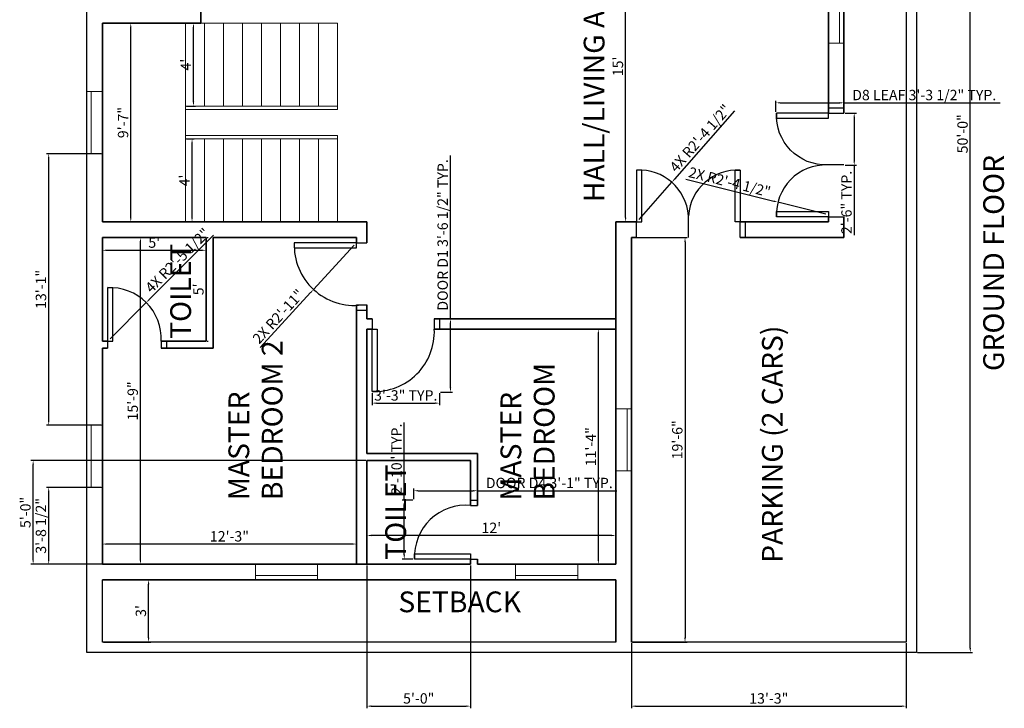
# Model space of a CAD drawing. Units: inches. Extents: x 2641 to 3210, y 2696 to 4064.
# Tile 1 of 4: x 2641 to 3210, y 2696 to 3095. Entities that reach past the tile are written whole.
import ezdxf

# ---------------------------------------------------------------- set-up
doc = ezdxf.new("R2010")
doc.units = ezdxf.units.IN
for name, color, linetype, lineweight in [('A-ANNO-DIMS', 2, 'Continuous', 18), ('A-ANNO-TEXT', 7, 'Continuous', 25), ('A-AREA-IDEN', 7, 'Continuous', 18), ('A-DOOR', 3, 'Continuous', 25), ('A-FLOR-STRS', 7, 'Continuous', 18), ('A-GLAZ', 4, 'Continuous', 18), ('A-WALL', 7, 'Continuous', 35), ('C-PROP', 8, 'Continuous', 25)]:
    doc.layers.add(name, color=color, linetype=linetype, lineweight=lineweight)
doc.styles.get("Standard").update_dxf_attribs({"font": 'arial.ttf'})
doc.dimstyles.new('ISO-25', dxfattribs={"dimtxt": 6, "dimasz": 2.5, "dimexe": 1.25, "dimexo": 0.625, "dimtad": 1, "dimdec": 1, "dimlunit": 3, "dimtxsty": 'Standard', "dimcen": 2.5, "dimadec": 0, "dimazin": 0, "dimtfac": 1, "dimtdec": 1, "dimtmove": 0, "dimatfit": 3, "dimfxl": 1, "dimarcsym": 0})

# ---------------------------------------------------------------- blocks, each defined once
blk = doc.blocks.new('*D2')
at = {"layer": 'A-ANNO-DIMS', "color": 0, "lineweight": -2, "transparency": 16777216}
for p, q in [((2689.25, 2968.55), (2711.9, 2968.55)), ((2710.65, 2782.05), (2710.65, 2966.05)), ((2689.25, 2779.55), (2711.9, 2779.55))]:
    blk.add_line(p, q, dxfattribs=at)
at = {"layer": 'A-ANNO-DIMS', "color": 0, "transparency": 16777216}
for points in [[(2710.23, 2966.05), (2711.06, 2966.05), (2710.65, 2968.55)], [(2710.23, 2782.05), (2711.06, 2782.05), (2710.65, 2779.55)]]:
    blk.add_solid(points, dxfattribs=at)
at = {"layer": 'Defpoints', "color": 0, "transparency": 16777216}
for p in [(2688.63, 2968.55), (2710.65, 2968.55), (2688.63, 2779.55)]:
    blk.add_point(p, dxfattribs=at)
at = {"layer": 'A-ANNO-DIMS', "color": 0, "transparency": 16777216, "insert": (2706.96, 2874.05), "char_height": 6, "attachment_point": 5, "rotation": 90}
blk.add_mtext('15\'-9"', dxfattribs=at)
blk = doc.blocks.new('*D3')
at = {"layer": 'A-ANNO-DIMS', "color": 0, "lineweight": -2, "transparency": 16777216}
for p, q in [((2688.63, 2780.17), (2688.63, 2792.51)), ((2833.13, 2791.26), (2691.13, 2791.26)), ((2835.63, 2780.17), (2835.63, 2792.51))]:
    blk.add_line(p, q, dxfattribs=at)
at = {"layer": 'A-ANNO-DIMS', "color": 0, "transparency": 16777216}
for points in [[(2691.13, 2791.68), (2691.13, 2790.85), (2688.63, 2791.26)], [(2833.13, 2791.68), (2833.13, 2790.85), (2835.63, 2791.26)]]:
    blk.add_solid(points, dxfattribs=at)
at = {"layer": 'Defpoints', "color": 0, "transparency": 16777216}
for p in [(2688.63, 2791.26), (2688.63, 2779.55), (2835.63, 2779.55)]:
    blk.add_point(p, dxfattribs=at)
at = {"layer": 'A-ANNO-DIMS', "color": 0, "transparency": 16777216, "insert": (2762.13, 2794.95), "char_height": 6, "attachment_point": 5}
blk.add_mtext('12\'-3"', dxfattribs=at)
blk = doc.blocks.new('*D4')
at = {"layer": 'A-ANNO-DIMS', "color": 0, "lineweight": -2, "transparency": 16777216}
for p, q in [((2841.63, 2780.17), (2841.63, 2797.47)), ((2985.63, 2780.17), (2985.63, 2797.47)), ((2983.13, 2796.22), (2844.13, 2796.22))]:
    blk.add_line(p, q, dxfattribs=at)
at = {"layer": 'A-ANNO-DIMS', "color": 0, "transparency": 16777216}
for points in [[(2844.13, 2796.64), (2844.13, 2795.8), (2841.63, 2796.22)], [(2983.13, 2796.64), (2983.13, 2795.8), (2985.63, 2796.22)]]:
    blk.add_solid(points, dxfattribs=at)
at = {"layer": 'Defpoints', "color": 0, "transparency": 16777216}
for p in [(2841.63, 2796.22), (2841.63, 2779.55), (2985.63, 2779.55)]:
    blk.add_point(p, dxfattribs=at)
at = {"layer": 'A-ANNO-DIMS', "color": 0, "transparency": 16777216, "insert": (2913.63, 2799.86), "char_height": 6, "attachment_point": 5}
blk.add_mtext("12'", dxfattribs=at)
blk = doc.blocks.new('*D5')
at = {"layer": 'A-ANNO-DIMS', "color": 0, "lineweight": -2, "transparency": 16777216}
for p, q in [((2985, 2915.55), (2974.29, 2915.55)), ((2975.54, 2782.05), (2975.54, 2913.05)), ((2985, 2779.55), (2974.29, 2779.55))]:
    blk.add_line(p, q, dxfattribs=at)
at = {"layer": 'A-ANNO-DIMS', "color": 0, "transparency": 16777216}
for points in [[(2975.13, 2913.05), (2975.96, 2913.05), (2975.54, 2915.55)], [(2975.13, 2782.05), (2975.96, 2782.05), (2975.54, 2779.55)]]:
    blk.add_solid(points, dxfattribs=at)
at = {"layer": 'Defpoints', "color": 0, "transparency": 16777216}
for p in [(2975.54, 2915.55), (2985.63, 2915.55), (2985.63, 2779.55)]:
    blk.add_point(p, dxfattribs=at)
at = {"layer": 'A-ANNO-DIMS', "color": 0, "transparency": 16777216, "insert": (2971.91, 2847.55), "char_height": 6, "attachment_point": 5, "rotation": 90}
blk.add_mtext('11\'-4"', dxfattribs=at)
blk = doc.blocks.new('*D6')
at = {"layer": 'A-ANNO-DIMS', "color": 0, "lineweight": -2, "transparency": 16777216}
for p, q in [((2749.25, 2968.55), (2749.88, 2968.55)), ((2748.63, 2911.05), (2748.63, 2966.05)), ((2749.25, 2908.55), (2749.88, 2908.55))]:
    blk.add_line(p, q, dxfattribs=at)
at = {"layer": 'A-ANNO-DIMS', "color": 0, "transparency": 16777216}
for points in [[(2748.21, 2966.05), (2749.04, 2966.05), (2748.63, 2968.55)], [(2748.21, 2911.05), (2749.04, 2911.05), (2748.63, 2908.55)]]:
    blk.add_solid(points, dxfattribs=at)
at = {"layer": 'Defpoints', "color": 0, "transparency": 16777216}
for p in [(2748.63, 2968.55), (2748.63, 2968.55), (2748.63, 2908.55)]:
    blk.add_point(p, dxfattribs=at)
at = {"layer": 'A-ANNO-DIMS', "color": 0, "transparency": 16777216, "insert": (2744.95, 2938.55), "char_height": 6, "attachment_point": 5, "rotation": 90}
blk.add_mtext("5'", dxfattribs=at)
blk = doc.blocks.new('*D7')
at = {"layer": 'A-ANNO-DIMS', "color": 0, "lineweight": -2, "transparency": 16777216}
for p, q in [((2688.63, 2967.92), (2688.63, 2959.92)), ((2748.63, 2967.92), (2748.63, 2959.92)), ((2691.13, 2961.17), (2746.13, 2961.17))]:
    blk.add_line(p, q, dxfattribs=at)
at = {"layer": 'A-ANNO-DIMS', "color": 0, "transparency": 16777216}
for points in [[(2691.13, 2961.59), (2691.13, 2960.76), (2688.63, 2961.17)], [(2746.13, 2961.59), (2746.13, 2960.76), (2748.63, 2961.17)]]:
    blk.add_solid(points, dxfattribs=at)
at = {"layer": 'Defpoints', "color": 0, "transparency": 16777216}
for p in [(2688.63, 2968.55), (2748.63, 2968.55), (2748.63, 2961.17)]:
    blk.add_point(p, dxfattribs=at)
at = {"layer": 'A-ANNO-DIMS', "color": 0, "transparency": 16777216, "insert": (2718.63, 2964.85), "char_height": 6, "attachment_point": 5}
blk.add_mtext("5'", dxfattribs=at)
blk = doc.blocks.new('*D14')
at = {"layer": 'A-ANNO-DIMS', "color": 0, "lineweight": -2, "transparency": 16777216}
for p, q in [((2991, 3157.55), (2990.07, 3157.55)), ((2991.32, 2980.05), (2991.32, 3155.05)), ((2991, 2977.55), (2990.07, 2977.55))]:
    blk.add_line(p, q, dxfattribs=at)
at = {"layer": 'A-ANNO-DIMS', "color": 0, "transparency": 16777216}
for points in [[(2990.9, 3155.05), (2991.74, 3155.05), (2991.32, 3157.55)], [(2990.9, 2980.05), (2991.74, 2980.05), (2991.32, 2977.55)]]:
    blk.add_solid(points, dxfattribs=at)
at = {"layer": 'Defpoints', "color": 0, "transparency": 16777216}
for p in [(2991.32, 3157.55), (2991.63, 3157.55), (2991.63, 2977.55)]:
    blk.add_point(p, dxfattribs=at)
at = {"layer": 'A-ANNO-DIMS', "color": 0, "transparency": 16777216, "insert": (2987.63, 3067.55), "char_height": 6, "attachment_point": 5, "rotation": 90}
blk.add_mtext("15'", dxfattribs=at)
blk = doc.blocks.new('*D15')
at = {"layer": 'A-ANNO-DIMS', "color": 0, "lineweight": -2, "transparency": 16777216}
for p, q in [((2689.25, 3092.55), (2706.31, 3092.55)), ((2705.06, 2980.05), (2705.06, 3090.05)), ((2689.25, 2977.55), (2706.31, 2977.55))]:
    blk.add_line(p, q, dxfattribs=at)
at = {"layer": 'A-ANNO-DIMS', "color": 0, "transparency": 16777216}
for points in [[(2704.64, 3090.05), (2705.47, 3090.05), (2705.06, 3092.55)], [(2704.64, 2980.05), (2705.47, 2980.05), (2705.06, 2977.55)]]:
    blk.add_solid(points, dxfattribs=at)
at = {"layer": 'Defpoints', "color": 0, "transparency": 16777216}
for p in [(2688.63, 3092.55), (2705.06, 3092.55), (2688.63, 2977.55)]:
    blk.add_point(p, dxfattribs=at)
at = {"layer": 'A-ANNO-DIMS', "color": 0, "transparency": 16777216, "insert": (2701.37, 3035.05), "char_height": 6, "attachment_point": 5, "rotation": 90}
blk.add_mtext('9\'-7"', dxfattribs=at)
blk = doc.blocks.new('*D16')
at = {"layer": 'A-ANNO-DIMS', "color": 0, "lineweight": -2, "transparency": 16777216}
for p, q in [((2737.25, 3025.55), (2741.74, 3025.55)), ((2740.49, 2980.05), (2740.49, 3023.05)), ((2737.25, 2977.55), (2741.74, 2977.55))]:
    blk.add_line(p, q, dxfattribs=at)
at = {"layer": 'A-ANNO-DIMS', "color": 0, "transparency": 16777216}
for points in [[(2740.08, 3023.05), (2740.91, 3023.05), (2740.49, 3025.55)], [(2740.08, 2980.05), (2740.91, 2980.05), (2740.49, 2977.55)]]:
    blk.add_solid(points, dxfattribs=at)
at = {"layer": 'Defpoints', "color": 0, "transparency": 16777216}
for p in [(2736.63, 3025.55), (2740.49, 3025.55), (2736.63, 2977.55)]:
    blk.add_point(p, dxfattribs=at)
at = {"layer": 'A-ANNO-DIMS', "color": 0, "transparency": 16777216, "insert": (2736.87, 3001.55), "char_height": 6, "attachment_point": 5, "rotation": 90}
blk.add_mtext("4'", dxfattribs=at)
blk = doc.blocks.new('*D17')
at = {"layer": 'A-ANNO-DIMS', "color": 0, "lineweight": -2, "transparency": 16777216}
for p, q in [((2737.25, 3092.55), (2742.57, 3092.55)), ((2741.32, 3047.05), (2741.32, 3090.05)), ((2737.25, 3044.55), (2742.57, 3044.55))]:
    blk.add_line(p, q, dxfattribs=at)
at = {"layer": 'A-ANNO-DIMS', "color": 0, "transparency": 16777216}
for points in [[(2740.9, 3090.05), (2741.73, 3090.05), (2741.32, 3092.55)], [(2740.9, 3047.05), (2741.73, 3047.05), (2741.32, 3044.55)]]:
    blk.add_solid(points, dxfattribs=at)
at = {"layer": 'Defpoints', "color": 0, "transparency": 16777216}
for p in [(2736.63, 3092.55), (2741.32, 3092.55), (2736.63, 3044.55)]:
    blk.add_point(p, dxfattribs=at)
at = {"layer": 'A-ANNO-DIMS', "color": 0, "transparency": 16777216, "insert": (2737.69, 3068.55), "char_height": 6, "attachment_point": 5, "rotation": 90}
blk.add_mtext("4'", dxfattribs=at)
blk = doc.blocks.new('*D18')
at = {"layer": 'A-ANNO-DIMS', "color": 0, "lineweight": -2, "transparency": 16777216}
for p, q in [((2689.25, 2770.55), (2716.61, 2770.55)), ((2715.36, 2737.05), (2715.36, 2768.05)), ((2689.25, 2734.55), (2716.61, 2734.55))]:
    blk.add_line(p, q, dxfattribs=at)
at = {"layer": 'A-ANNO-DIMS', "color": 0, "transparency": 16777216}
for points in [[(2714.94, 2768.05), (2715.78, 2768.05), (2715.36, 2770.55)], [(2714.94, 2737.05), (2715.78, 2737.05), (2715.36, 2734.55)]]:
    blk.add_solid(points, dxfattribs=at)
at = {"layer": 'Defpoints', "color": 0, "transparency": 16777216}
for p in [(2688.63, 2770.55), (2715.36, 2770.55), (2688.63, 2734.55)]:
    blk.add_point(p, dxfattribs=at)
at = {"layer": 'A-ANNO-DIMS', "color": 0, "transparency": 16777216, "insert": (2711.67, 2752.55), "char_height": 6, "attachment_point": 5, "rotation": 90}
blk.add_mtext("3'", dxfattribs=at)
blk = doc.blocks.new('DOOR-36-INT')
for p, q in [((0, 42.03), (0, 36.03)), ((36, 42.03), (36, 36.03)), ((39, 42.03), (39, 36.03))]:
    blk.add_line(p, q)
blk.add_lwpolyline([(0, 36.03), (3, 36.03), (3, 0.03), (0, 0.03)], close=True)
blk.add_arc((1.5, 34.53), 34.53, 267.5104, 2.4896)
blk = doc.blocks.new('DOOR-60-PAIR')
for p, q in [((30, 0), (30, 12.64)), ((0, 0), (0, 9)), ((60, 0), (60, 9)), ((63, 0), (63, 9))]:
    blk.add_line(p, q)
for points in [[(0, 9), (3, 9), (3, 39), (0, 39)], [(60, 9), (57, 9), (57, 39), (60, 39)]]:
    blk.add_lwpolyline(points, close=True)
for centre, start, end in [((1.5, 10.46), 4.3856, 93.0081), ((58.5, 10.46), 86.9919, 175.6144)]:
    blk.add_arc(centre, 28.58, start, end)
blk = doc.blocks.new('DOOR-36-BEDROOM')
for p, q in [((36.03, 39), (42.03, 39)), ((36.03, 3), (42.03, 3)), ((36.03, 0), (42.03, 0))]:
    blk.add_line(p, q)
blk.add_lwpolyline([(36.03, 39), (0.03, 39), (0.03, 36), (36.03, 36)], close=True)
blk.add_arc((34.76, 37.5), 34.76, 177.527, 277.0543)
blk = doc.blocks.new('DOOR-BATH-32P4')
for p, q in [((32.44, 34), (36.44, 34)), ((32.44, 31), (36.44, 31)), ((32.44, 0), (36.44, 0))]:
    blk.add_line(p, q)
blk.add_lwpolyline([(32.44, 0), (0.04, 0), (0.04, 3), (32.44, 3)], close=True)
blk.add_arc((29.63, 1.5), 29.63, 84.5685, 182.9015)
blk = doc.blocks.new('DOOR-31-BATH')
for p, q in [((0, 4), (0, 0)), ((31, 4), (31, 0)), ((34, 4), (34, 0))]:
    blk.add_line(p, q)
blk.add_lwpolyline([(0, 4), (3, 4), (3, 35), (0, 35)], close=True)
blk.add_arc((1.5, 5.5), 29.54, 357.0892, 92.9108)
blk = doc.blocks.new('DOOR-30-PAIRED-LEAF')
blk.add_line((30.04, 0), (39.04, 0))
blk.add_lwpolyline([(30.04, 0), (0.04, 0), (0.04, 3), (30.04, 3)], close=True)
blk.add_arc((28.51, 1.5), 28.51, 88.3458, 183.0157)
blk = doc.blocks.new('WIN-36x9')
blk.add_line((6.5, 36), (6.5, 0))
blk.add_lwpolyline([(9, 36), (0, 36), (0, 0), (9, 0)], close=True)
blk = doc.blocks.new('STAIR-RETURN-FLIGHTS')
for p, q in [((0, 0), (0, 115)), ((88, 115), (9, 115)), ((11, 67), (11, 115)), ((22, 67), (22, 115)), ((33, 67), (33, 115)), ((44, 67), (44, 115)), ((55, 67), (55, 115)), ((66, 67), (66, 115)), ((77, 67), (77, 115)), ((88, 67), (88, 115)), ((88, 67), (0, 67)), ((88, 65), (0, 65)), ((88, 65), (88, 67)), ((88, 50), (0, 50)), ((88, 48), (0, 48)), ((11, 0), (11, 48)), ((22, 0), (22, 48)), ((33, 0), (33, 48)), ((44, 0), (44, 48)), ((55, 0), (55, 48)), ((66, 0), (66, 48)), ((77, 0), (77, 48)), ((88, 48), (88, 50)), ((88, 0), (88, 48))]:
    blk.add_line(p, q)
blk = doc.blocks.new('*D33')
at = {"layer": 'A-ANNO-DIMS', "color": 0, "lineweight": -2, "transparency": 16777216}
for p, q in [((2889.99, 2921.55), (2889.99, 3016.07)), ((2884.25, 2921.55), (2891.24, 2921.55)), ((2889.99, 2881.63), (2889.99, 2919.05)), ((2884.25, 2879.13), (2891.24, 2879.13))]:
    blk.add_line(p, q, dxfattribs=at)
at = {"layer": 'A-ANNO-DIMS', "color": 0, "transparency": 16777216}
for points in [[(2889.57, 2919.05), (2890.41, 2919.05), (2889.99, 2921.55)], [(2889.57, 2881.63), (2890.41, 2881.63), (2889.99, 2879.13)]]:
    blk.add_solid(points, dxfattribs=at)
at = {"layer": 'Defpoints', "color": 0, "transparency": 16777216}
for p in [(2883.63, 2921.55), (2889.99, 2921.55), (2883.63, 2879.13)]:
    blk.add_point(p, dxfattribs=at)
at = {"layer": 'A-ANNO-DIMS', "color": 0, "transparency": 16777216, "insert": (2886.26, 2970.06), "char_height": 6, "attachment_point": 5, "rotation": 90}
blk.add_mtext('DOOR D1 3\'-6 1/2" TYP.', dxfattribs=at)
blk = doc.blocks.new('*D34')
at = {"layer": 'A-ANNO-DIMS', "color": 0, "lineweight": -2, "transparency": 16777216}
for p, q in [((2844.63, 2878.5), (2844.63, 2871.52)), ((2883.63, 2878.5), (2883.63, 2871.52)), ((2847.13, 2872.77), (2881.13, 2872.77))]:
    blk.add_line(p, q, dxfattribs=at)
at = {"layer": 'A-ANNO-DIMS', "color": 0, "transparency": 16777216}
for points in [[(2847.13, 2873.18), (2847.13, 2872.35), (2844.63, 2872.77)], [(2881.13, 2873.18), (2881.13, 2872.35), (2883.63, 2872.77)]]:
    blk.add_solid(points, dxfattribs=at)
at = {"layer": 'Defpoints', "color": 0, "transparency": 16777216}
for p in [(2844.63, 2879.13), (2883.63, 2879.13), (2883.63, 2872.77)]:
    blk.add_point(p, dxfattribs=at)
at = {"layer": 'A-ANNO-DIMS', "color": 0, "transparency": 16777216, "insert": (2864.13, 2876.46), "char_height": 6, "attachment_point": 5}
blk.add_mtext('3\'-3" TYP.', dxfattribs=at)
blk = doc.blocks.new('*D39')
at = {"layer": 'A-ANNO-DIMS', "color": 0, "lineweight": -2, "transparency": 16777216}
for p, q in [((2868.79, 2817.17), (2868.79, 2823.33)), ((2871.29, 2822.08), (2903.13, 2822.08)), ((2905.63, 2817.17), (2905.63, 2823.33)), ((2905.63, 2822.08), (2986.17, 2822.08))]:
    blk.add_line(p, q, dxfattribs=at)
at = {"layer": 'A-ANNO-DIMS', "color": 0, "transparency": 16777216}
for points in [[(2871.29, 2822.49), (2871.29, 2821.66), (2868.79, 2822.08)], [(2903.13, 2822.49), (2903.13, 2821.66), (2905.63, 2822.08)]]:
    blk.add_solid(points, dxfattribs=at)
at = {"layer": 'Defpoints', "color": 0, "transparency": 16777216}
for p in [(2905.63, 2822.08), (2868.79, 2816.55), (2905.63, 2816.55)]:
    blk.add_point(p, dxfattribs=at)
at = {"layer": 'A-ANNO-DIMS', "color": 0, "transparency": 16777216, "insert": (2947.15, 2825.81), "char_height": 6, "attachment_point": 5}
blk.add_mtext('DOOR D4 3\'-1" TYP.', dxfattribs=at)
blk = doc.blocks.new('*D40')
at = {"layer": 'A-ANNO-DIMS', "color": 0, "lineweight": -2, "transparency": 16777216}
for p, q in [((2863.26, 2816.55), (2863.26, 2861.64)), ((2868.17, 2816.55), (2862.01, 2816.55)), ((2863.26, 2785.05), (2863.26, 2814.05)), ((2868.17, 2782.55), (2862.01, 2782.55))]:
    blk.add_line(p, q, dxfattribs=at)
at = {"layer": 'A-ANNO-DIMS', "color": 0, "transparency": 16777216}
for points in [[(2862.85, 2814.05), (2863.68, 2814.05), (2863.26, 2816.55)], [(2862.85, 2785.05), (2863.68, 2785.05), (2863.26, 2782.55)]]:
    blk.add_solid(points, dxfattribs=at)
at = {"layer": 'Defpoints', "color": 0, "transparency": 16777216}
for p in [(2863.26, 2816.55), (2868.79, 2816.55), (2868.79, 2782.55)]:
    blk.add_point(p, dxfattribs=at)
at = {"layer": 'A-ANNO-DIMS', "color": 0, "transparency": 16777216, "insert": (2859.58, 2840.34), "char_height": 6, "attachment_point": 5, "rotation": 90}
blk.add_mtext('2\'-10" TYP.', dxfattribs=at)
blk = doc.blocks.new('*D47')
at = {"layer": 'A-ANNO-DIMS', "color": 0, "lineweight": -2, "transparency": 16777216}
for p, q in [((3078.21, 3041.17), (3078.21, 3047.71)), ((3117.63, 3041.17), (3117.63, 3047.71)), ((3080.71, 3046.46), (3115.13, 3046.46)), ((3117.63, 3046.46), (3207.97, 3046.46))]:
    blk.add_line(p, q, dxfattribs=at)
at = {"layer": 'A-ANNO-DIMS', "color": 0, "transparency": 16777216}
for points in [[(3080.71, 3046.88), (3080.71, 3046.05), (3078.21, 3046.46)], [(3115.13, 3046.88), (3115.13, 3046.05), (3117.63, 3046.46)]]:
    blk.add_solid(points, dxfattribs=at)
at = {"layer": 'Defpoints', "color": 0, "transparency": 16777216}
for p in [(3117.63, 3046.46), (3078.21, 3040.55), (3117.63, 3040.55)]:
    blk.add_point(p, dxfattribs=at)
at = {"layer": 'A-ANNO-DIMS', "color": 0, "transparency": 16777216, "insert": (3164.05, 3050.19), "char_height": 6, "attachment_point": 5}
blk.add_mtext('D8 LEAF 3\'-3 1/2" TYP.', dxfattribs=at)
blk = doc.blocks.new('*D48')
at = {"layer": 'A-ANNO-DIMS', "color": 0, "lineweight": -2, "transparency": 16777216}
for p, q in [((3118.25, 3040.55), (3124.79, 3040.55)), ((3123.54, 3038.05), (3123.54, 3012.82)), ((3118.25, 3010.32), (3124.79, 3010.32)), ((3123.54, 3010.32), (3123.54, 2969.89))]:
    blk.add_line(p, q, dxfattribs=at)
at = {"layer": 'A-ANNO-DIMS', "color": 0, "transparency": 16777216}
for points in [[(3123.12, 3038.05), (3123.96, 3038.05), (3123.54, 3040.55)], [(3123.12, 3012.82), (3123.96, 3012.82), (3123.54, 3010.32)]]:
    blk.add_solid(points, dxfattribs=at)
at = {"layer": 'Defpoints', "color": 0, "transparency": 16777216}
for p in [(3117.63, 3040.55), (3117.63, 3010.32), (3123.54, 3010.32)]:
    blk.add_point(p, dxfattribs=at)
at = {"layer": 'A-ANNO-DIMS', "color": 0, "transparency": 16777216, "insert": (3119.85, 2988.86), "char_height": 6, "attachment_point": 5, "rotation": 90}
blk.add_mtext('2\'-6" TYP.', dxfattribs=at)
blk = doc.blocks.new('*D52')
at = {"layer": 'A-ANNO-DIMS', "color": 0, "lineweight": -2, "transparency": 16777216}
for p, q in [((3160.25, 3328.55), (3191.93, 3328.55)), ((3190.68, 2731.05), (3190.68, 3326.05)), ((3160.25, 2728.55), (3191.93, 2728.55))]:
    blk.add_line(p, q, dxfattribs=at)
at = {"layer": 'A-ANNO-DIMS', "color": 0, "transparency": 16777216}
for points in [[(3190.26, 3326.05), (3191.09, 3326.05), (3190.68, 3328.55)], [(3190.26, 2731.05), (3191.09, 2731.05), (3190.68, 2728.55)]]:
    blk.add_solid(points, dxfattribs=at)
at = {"layer": 'Defpoints', "color": 0, "transparency": 16777216}
for p in [(3159.63, 3328.55), (3190.68, 3328.55), (3159.63, 2728.55)]:
    blk.add_point(p, dxfattribs=at)
at = {"layer": 'A-ANNO-DIMS', "color": 0, "transparency": 16777216, "insert": (3186.99, 3028.55), "char_height": 6, "attachment_point": 5, "rotation": 90}
blk.add_mtext('50\'-0"', dxfattribs=at)
blk = doc.blocks.new('*D53')
at = {"layer": 'A-ANNO-DIMS', "color": 0, "lineweight": -2, "transparency": 16777216}
for p, q in [((2994.63, 2733.92), (2994.63, 2696.25)), ((3153.63, 2733.92), (3153.63, 2696.25)), ((2997.13, 2697.5), (3151.13, 2697.5))]:
    blk.add_line(p, q, dxfattribs=at)
at = {"layer": 'A-ANNO-DIMS', "color": 0, "transparency": 16777216}
for points in [[(2997.13, 2697.92), (2997.13, 2697.08), (2994.63, 2697.5)], [(3151.13, 2697.92), (3151.13, 2697.08), (3153.63, 2697.5)]]:
    blk.add_solid(points, dxfattribs=at)
at = {"layer": 'Defpoints', "color": 0, "transparency": 16777216}
for p in [(2994.63, 2734.55), (3153.63, 2734.55), (3153.63, 2697.5)]:
    blk.add_point(p, dxfattribs=at)
at = {"layer": 'A-ANNO-DIMS', "color": 0, "transparency": 16777216, "insert": (3074.13, 2701.19), "char_height": 6, "attachment_point": 5}
blk.add_mtext('13\'-3"', dxfattribs=at)
blk = doc.blocks.new('*D54')
at = {"layer": 'A-ANNO-DIMS', "color": 0, "lineweight": -2, "transparency": 16777216}
for p, q in [((2995.25, 2968.55), (3026.93, 2968.55)), ((3025.68, 2966.05), (3025.68, 2737.05)), ((2995.25, 2734.55), (3026.93, 2734.55))]:
    blk.add_line(p, q, dxfattribs=at)
at = {"layer": 'A-ANNO-DIMS', "color": 0, "transparency": 16777216}
for points in [[(3025.26, 2966.05), (3026.09, 2966.05), (3025.68, 2968.55)], [(3025.26, 2737.05), (3026.09, 2737.05), (3025.68, 2734.55)]]:
    blk.add_solid(points, dxfattribs=at)
at = {"layer": 'Defpoints', "color": 0, "transparency": 16777216}
for p in [(2994.63, 2968.55), (2994.63, 2734.55), (3025.68, 2734.55)]:
    blk.add_point(p, dxfattribs=at)
at = {"layer": 'A-ANNO-DIMS', "color": 0, "transparency": 16777216, "insert": (3021.99, 2851.55), "char_height": 6, "attachment_point": 5, "rotation": 90}
blk.add_mtext('19\'-6"', dxfattribs=at)
blk = doc.blocks.new('*D55')
at = {"layer": 'A-ANNO-DIMS', "color": 0, "lineweight": -2, "transparency": 16777216}
for p, q in [((2841.63, 2778.92), (2841.63, 2696.25)), ((2901.63, 2778.92), (2901.63, 2696.25)), ((2844.13, 2697.5), (2899.13, 2697.5))]:
    blk.add_line(p, q, dxfattribs=at)
at = {"layer": 'A-ANNO-DIMS', "color": 0, "transparency": 16777216}
for points in [[(2844.13, 2697.92), (2844.13, 2697.08), (2841.63, 2697.5)], [(2899.13, 2697.92), (2899.13, 2697.08), (2901.63, 2697.5)]]:
    blk.add_solid(points, dxfattribs=at)
at = {"layer": 'Defpoints', "color": 0, "transparency": 16777216}
for p in [(2841.63, 2779.55), (2901.63, 2779.55), (2901.63, 2697.5)]:
    blk.add_point(p, dxfattribs=at)
at = {"layer": 'A-ANNO-DIMS', "color": 0, "transparency": 16777216, "insert": (2871.63, 2701.19), "char_height": 6, "attachment_point": 5}
blk.add_mtext('5\'-0"', dxfattribs=at)
blk = doc.blocks.new('*D56')
at = {"layer": 'A-ANNO-DIMS', "color": 0, "lineweight": -2, "transparency": 16777216}
for p, q in [((2841, 2839.55), (2647.33, 2839.55)), ((2648.58, 2782.05), (2648.58, 2837.05)), ((2841, 2779.55), (2647.33, 2779.55))]:
    blk.add_line(p, q, dxfattribs=at)
at = {"layer": 'A-ANNO-DIMS', "color": 0, "transparency": 16777216}
for points in [[(2648.16, 2837.05), (2648.99, 2837.05), (2648.58, 2839.55)], [(2648.16, 2782.05), (2648.99, 2782.05), (2648.58, 2779.55)]]:
    blk.add_solid(points, dxfattribs=at)
at = {"layer": 'Defpoints', "color": 0, "transparency": 16777216}
for p in [(2648.58, 2839.55), (2841.63, 2839.55), (2841.63, 2779.55)]:
    blk.add_point(p, dxfattribs=at)
at = {"layer": 'A-ANNO-DIMS', "color": 0, "transparency": 16777216, "insert": (2644.89, 2809.55), "char_height": 6, "attachment_point": 5, "rotation": 90}
blk.add_mtext('5\'-0"', dxfattribs=at)
blk = doc.blocks.new('*D64')
at = {"layer": 'A-ANNO-DIMS', "color": 0, "lineweight": -2, "transparency": 16777216}
for p, q in [((2688, 2824.05), (2656.33, 2824.05)), ((2657.58, 2782.05), (2657.58, 2821.55)), ((2688, 2779.55), (2656.33, 2779.55))]:
    blk.add_line(p, q, dxfattribs=at)
at = {"layer": 'A-ANNO-DIMS', "color": 0, "transparency": 16777216}
for points in [[(2657.16, 2821.55), (2657.99, 2821.55), (2657.58, 2824.05)], [(2657.16, 2782.05), (2657.99, 2782.05), (2657.58, 2779.55)]]:
    blk.add_solid(points, dxfattribs=at)
at = {"layer": 'Defpoints', "color": 0, "transparency": 16777216}
for p in [(2657.58, 2824.05), (2688.63, 2824.05), (2688.63, 2779.55)]:
    blk.add_point(p, dxfattribs=at)
at = {"layer": 'A-ANNO-DIMS', "color": 0, "transparency": 16777216, "insert": (2653.85, 2801.8), "char_height": 6, "attachment_point": 5, "rotation": 90}
blk.add_mtext('3\'-8 1/2"', dxfattribs=at)
blk = doc.blocks.new('*D65')
at = {"layer": 'A-ANNO-DIMS', "color": 0, "lineweight": -2, "transparency": 16777216}
for p, q in [((2688, 3017.05), (2656.33, 3017.05)), ((2657.58, 2862.55), (2657.58, 3014.55)), ((2688, 2860.05), (2656.33, 2860.05))]:
    blk.add_line(p, q, dxfattribs=at)
at = {"layer": 'A-ANNO-DIMS', "color": 0, "transparency": 16777216}
for points in [[(2657.16, 3014.55), (2657.99, 3014.55), (2657.58, 3017.05)], [(2657.16, 2862.55), (2657.99, 2862.55), (2657.58, 2860.05)]]:
    blk.add_solid(points, dxfattribs=at)
at = {"layer": 'Defpoints', "color": 0, "transparency": 16777216}
for p in [(2657.58, 3017.05), (2688.63, 3017.05), (2688.63, 2860.05)]:
    blk.add_point(p, dxfattribs=at)
at = {"layer": 'A-ANNO-DIMS', "color": 0, "transparency": 16777216, "insert": (2653.89, 2938.55), "char_height": 6, "attachment_point": 5, "rotation": 90}
blk.add_mtext('13\'-1"', dxfattribs=at)
blk = doc.blocks.new('*D85')
at = {"layer": 'A-ANNO-DIMS', "color": 0, "lineweight": -2, "transparency": 16777216}
for p, q in [((2834.36, 2964.05), (2810.78, 2938.51)), ((2779.85, 2905), (2809.08, 2936.67))]:
    blk.add_line(p, q, dxfattribs=at)
at = {"layer": 'A-ANNO-DIMS', "color": 0, "transparency": 16777216}
blk.add_solid([(2808.78, 2936.95), (2809.39, 2936.39), (2810.78, 2938.51)], dxfattribs=at)
at = {"layer": 'Defpoints', "color": 0, "transparency": 16777216}
for p in [(2834.36, 2964.05), (2810.78, 2938.51)]:
    blk.add_point(p, dxfattribs=at)
at = {"layer": 'A-ANNO-DIMS', "color": 0, "transparency": 16777216, "insert": (2790.94, 2922.39), "char_height": 6, "attachment_point": 5, "rotation": 47.2896}
blk.add_mtext('2X R2\'-11"', dxfattribs=at)
blk = doc.blocks.new('*D89')
at = {"layer": 'A-ANNO-DIMS', "color": 0, "lineweight": -2, "transparency": 16777216}
for p, q in [((2752.94, 2969.87), (2715.78, 2932.7)), ((2693.13, 2910.05), (2714.01, 2930.94))]:
    blk.add_line(p, q, dxfattribs=at)
at = {"layer": 'A-ANNO-DIMS', "color": 0, "transparency": 16777216}
blk.add_solid([(2715.49, 2933), (2716.07, 2932.41), (2714.01, 2930.94)], dxfattribs=at)
at = {"layer": 'Defpoints', "color": 0, "transparency": 16777216}
for p in [(2714.01, 2930.94), (2693.13, 2910.05)]:
    blk.add_point(p, dxfattribs=at)
at = {"layer": 'A-ANNO-DIMS', "color": 0, "transparency": 16777216, "insert": (2732.61, 2954.81), "char_height": 6, "attachment_point": 5, "rotation": 45.0002}
blk.add_mtext('4X R2\'-5 1/2"', dxfattribs=at)
blk = doc.blocks.new('*D90')
at = {"layer": 'A-ANNO-DIMS', "color": 0, "lineweight": -2, "transparency": 16777216}
for p, q in [((3054.33, 3041.84), (3019.64, 3002.36)), ((2999.13, 2979.01), (3017.99, 3000.48))]:
    blk.add_line(p, q, dxfattribs=at)
at = {"layer": 'A-ANNO-DIMS', "color": 0, "transparency": 16777216}
blk.add_solid([(3019.33, 3002.63), (3019.96, 3002.08), (3017.99, 3000.48)], dxfattribs=at)
at = {"layer": 'Defpoints', "color": 0, "transparency": 16777216}
for p in [(3017.99, 3000.48), (2999.13, 2979.01)]:
    blk.add_point(p, dxfattribs=at)
at = {"layer": 'A-ANNO-DIMS', "color": 0, "transparency": 16777216, "insert": (3035.01, 3025.5), "char_height": 6, "attachment_point": 5, "rotation": 48.697}
blk.add_mtext('4X R2\'-4 1/2"', dxfattribs=at)
blk = doc.blocks.new('*D91')
at = {"layer": 'A-ANNO-DIMS', "color": 0, "lineweight": -2, "transparency": 16777216}
for p, q in [((3026.18, 3002.36), (3077.02, 2989.6)), ((3107.1, 2982.05), (3079.44, 2988.99))]:
    blk.add_line(p, q, dxfattribs=at)
at = {"layer": 'A-ANNO-DIMS', "color": 0, "transparency": 16777216}
blk.add_solid([(3077.12, 2990), (3076.92, 2989.19), (3079.44, 2988.99)], dxfattribs=at)
at = {"layer": 'Defpoints', "color": 0, "transparency": 16777216}
for p in [(3079.44, 2988.99), (3107.1, 2982.05)]:
    blk.add_point(p, dxfattribs=at)
at = {"layer": 'A-ANNO-DIMS', "color": 0, "transparency": 16777216, "insert": (3051.29, 2999.9), "char_height": 6, "attachment_point": 5, "rotation": 345.9121}
blk.add_mtext('2X R2\'-4 1/2"', dxfattribs=at)

msp = doc.modelspace()

# ---------------------------------------------------------------- linework, layer by layer
at = {"layer": 'A-DOOR'}
for p, q in [((3108.63, 3043.55), (3117.63, 3043.55)), ((3117.63, 3010.55), (3107.92, 3010.55))]:
    msp.add_line(p, q, dxfattribs=at)
at = {"layer": 'A-WALL'}
for p, q in [((3108.63, 3157.55), (3108.63, 3040.55)), ((2745.63, 3092.55), (2745.63, 3099.55)), ((2688.63, 2977.55), (2688.63, 3092.55)), ((2688.63, 3092.55), (2745.63, 3092.55)), ((3108.63, 2977.55), (3108.63, 2980.55)), ((3108.63, 2980.55), (3108.63, 2977.55)), ((2841.63, 2977.55), (2688.63, 2977.55)), ((2841.63, 2977.55), (2841.63, 2965.55)), ((2985.63, 2977.55), (2985.63, 2929.55)), ((2997.63, 2977.55), (2985.63, 2977.55)), ((3108.63, 2977.55), (3057.63, 2977.55)), ((2688.63, 2908.55), (2688.63, 2968.55)), ((2748.63, 2968.55), (2688.63, 2968.55)), ((2748.63, 2908.55), (2748.63, 2968.55)), ((2835.63, 2968.55), (2752.63, 2968.55)), ((2752.63, 2904.55), (2752.63, 2968.55)), ((2835.63, 2968.55), (2835.63, 2965.55)), ((2835.63, 2968.55), (2835.63, 2965.55)), ((2994.63, 2968.55), (2994.63, 2734.55)), ((2994.63, 2968.55), (2997.63, 2968.55)), ((2997.63, 2968.55), (2994.63, 2968.55)), ((3117.63, 2968.55), (3057.63, 2968.55)), ((2835.63, 2929.55), (2835.63, 2779.55)), ((2841.63, 2929.55), (2841.63, 2921.55)), ((2985.63, 2923.55), (2985.63, 2929.55)), ((2985.63, 2923.55), (2985.63, 2779.55)), ((2841.63, 2921.55), (2844.63, 2921.55)), ((2841.63, 2921.55), (2844.63, 2921.55)), ((2880.63, 2921.55), (2985.63, 2921.55)), ((2841.63, 2915.55), (2844.63, 2915.55)), ((2841.63, 2915.55), (2841.63, 2843.55)), ((2880.63, 2915.55), (2985.63, 2915.55)), ((2688.63, 2908.55), (2691.63, 2908.55)), ((2691.63, 2908.55), (2688.63, 2908.55)), ((2748.63, 2908.55), (2722.63, 2908.55)), ((2688.63, 2779.55), (2688.63, 2904.55)), ((2691.63, 2904.55), (2688.63, 2904.55)), ((2752.63, 2904.55), (2722.63, 2904.55)), ((2905.63, 2843.55), (2841.63, 2843.55)), ((2905.63, 2843.55), (2905.63, 2813.55)), ((2901.63, 2839.55), (2841.63, 2839.55)), ((2841.63, 2839.55), (2841.63, 2779.55)), ((2901.63, 2839.55), (2901.63, 2813.55)), ((2901.63, 2779.55), (2688.63, 2779.55)), ((2901.63, 2779.55), (2901.63, 2782.55)), ((2901.63, 2782.55), (2901.63, 2779.55)), ((2905.63, 2782.55), (2905.63, 2779.55)), ((2985.63, 2779.55), (2905.63, 2779.55)), ((2985.63, 2770.55), (2985.63, 2734.55))]:
    msp.add_line(p, q, dxfattribs=at)
for points in [[(3105.63, 3286.55), (3117.63, 3286.55), (3117.63, 3040.55)], [(3117.63, 2980.55), (3117.63, 2968.55)], [(2985.63, 2770.55), (2688.63, 2770.55)]]:
    msp.add_lwpolyline(points, dxfattribs=at)
at = {"layer": 'C-PROP'}
for p, q in [((2679.63, 2728.55), (2679.63, 3328.55)), ((3159.63, 3328.55), (3159.63, 2728.55)), ((3153.63, 3322.55), (3153.63, 2968.55)), ((3153.63, 2968.55), (3153.63, 2734.55)), ((2688.63, 2734.55), (2688.63, 2770.55)), ((2985.63, 2734.55), (2688.63, 2734.55)), ((3153.63, 2734.55), (2994.63, 2734.55)), ((3159.63, 2728.55), (2679.63, 2728.55))]:
    msp.add_line(p, q, dxfattribs=at)

# ---------------------------------------------------------------- block references
at = {"layer": 'A-DOOR', "extrusion": (0, 0, -1), "zscale": -1, "rotation": 180}
msp.add_blockref('DOOR-30-PAIRED-LEAF', (-3078.59, 3040.55), dxfattribs=at)
at = {"layer": 'A-DOOR'}
for name, p in [('DOOR-60-PAIR', (2997.63, 2968.55)), ('DOOR-30-PAIRED-LEAF', (3078.59, 2980.55)), ('DOOR-36-BEDROOM', (2799.6, 2926.55)), ('DOOR-31-BATH', (2691.63, 2904.55)), ('DOOR-36-INT', (2844.63, 2879.52)), ('DOOR-BATH-32P4', (2869.19, 2782.55))]:
    msp.add_blockref(name, p, dxfattribs=at)
at = {"layer": 'A-FLOR-STRS'}
msp.add_blockref('STAIR-RETURN-FLIGHTS', (2736.63, 2977.55), dxfattribs=at)
at = {"layer": 'A-GLAZ'}
for p in [(3108.63, 3081.05), (2985.63, 2833.55)]:
    msp.add_blockref('WIN-36x9', p, dxfattribs=at)
for p, rotation in [((2688.63, 3053.05), 180), ((2688.63, 2860.05), 180), ((2777.13, 2779.55), 269.999999999999), ((2927.63, 2779.55), 269.9999999999982)]:
    msp.add_blockref('WIN-36x9', p, dxfattribs=dict(at, rotation=rotation))

# ---------------------------------------------------------------- texts
at = {"layer": 'A-ANNO-TEXT'}
msp.add_text('GROUND FLOOR', height=12, rotation=90, dxfattribs=at).set_placement((3210.16, 2891.33))
at = {"layer": 'A-AREA-IDEN'}
for s, p in [('HALL/LIVING AREA', (2979.08, 2988.98)), ('TOILET', (2739.91, 2909.92)), ('PARKING (2 CARS)', (3082.18, 2780.38)), ('BEDROOM 2', (2792.84, 2816.67)), ('BEDROOM', (2950.21, 2816.39)), ('MASTER', (2773.56, 2816.67)), ('MASTER', (2930.93, 2816.39)), ('TOILET', (2864.32, 2782.18))]:
    msp.add_text(s, height=12, rotation=90, dxfattribs=at).set_placement(p)
msp.add_text('SETBACK', height=12, dxfattribs=at).set_placement((2859.85, 2751.82))

# ---------------------------------------------------------------- dimensions: what is measured, and where the dimension line sits
at = {"layer": 'A-ANNO-DIMS'}
for base, p1, p2, angle, override, picture, middle in [((3190.68, 3328.55), (3159.63, 2728.55), (3159.63, 3328.55), 90, {"dimdec": 1, "dimlfac": 1, "dimrnd": 0, "dimzin": 1, "dimdsep": 46, "dimlunit": 4, "dimfrac": 2}, '*D52', (3186.99, 3028.55)), ((2991.32, 3157.55), (2991.63, 2977.55), (2991.63, 3157.55), 90, {"dimclrd": 0, "dimclre": 0, "dimclrt": 0}, '*D14', (2987.63, 3067.55)), ((2705.06, 3092.55), (2688.63, 2977.55), (2688.63, 3092.55), 90, {"dimclrd": 0, "dimclre": 0, "dimclrt": 0}, '*D15', (2701.37, 3035.05)), ((2741.32, 3092.55), (2736.63, 3044.55), (2736.63, 3092.55), 90, {"dimclrd": 0, "dimclre": 0, "dimclrt": 0}, '*D17', (2737.69, 3068.55)), ((2740.49, 3025.55), (2736.63, 2977.55), (2736.63, 3025.55), 90, {"dimclrd": 0, "dimclre": 0, "dimclrt": 0}, '*D16', (2736.87, 3001.55)), ((2657.58, 3017.05), (2688.63, 2860.05), (2688.63, 3017.05), 90, {"dimdec": 1, "dimlfac": 1, "dimrnd": 0, "dimzin": 1, "dimdsep": 46, "dimlunit": 4, "dimfrac": 2}, '*D65', (2653.89, 2938.55)), ((2710.65, 2968.55), (2688.63, 2779.55), (2688.63, 2968.55), 90, {"dimclrd": 0, "dimclre": 0, "dimclrt": 0}, '*D2', (2706.96, 2874.05)), ((2748.63, 2968.55), (2748.63, 2908.55), (2748.63, 2968.55), 90, {"dimclrd": 0, "dimclre": 0, "dimclrt": 0}, '*D6', (2744.95, 2938.55)), ((3025.68, 2734.55), (2994.63, 2968.55), (2994.63, 2734.55), 270, {"dimdec": 1, "dimlfac": 1, "dimrnd": 0, "dimzin": 1, "dimdsep": 46, "dimlunit": 4, "dimfrac": 2}, '*D54', (3021.99, 2851.55)), ((2975.54, 2915.55), (2985.63, 2779.55), (2985.63, 2915.55), 90, {"dimclrd": 0, "dimclre": 0, "dimclrt": 0}, '*D5', (2971.91, 2847.55)), ((2648.58, 2839.55), (2841.63, 2779.55), (2841.63, 2839.55), 90, {"dimdec": 1, "dimlfac": 1, "dimrnd": 0, "dimzin": 1, "dimdsep": 46, "dimlunit": 4, "dimfrac": 2}, '*D56', (2644.89, 2809.55)), ((2657.58, 2824.05), (2688.63, 2779.55), (2688.63, 2824.05), 90, {"dimdec": 1, "dimlfac": 1, "dimrnd": 0, "dimzin": 1, "dimdsep": 46, "dimlunit": 4, "dimfrac": 2}, '*D64', (2653.85, 2801.8)), ((2715.36, 2770.55), (2688.63, 2734.55), (2688.63, 2770.55), 90, {"dimclrd": 0, "dimclre": 0, "dimclrt": 0}, '*D18', (2711.67, 2752.55))]:
    dim = msp.add_linear_dim(base=base, p1=p1, p2=p2, angle=angle, dimstyle='ISO-25', override=override, dxfattribs=at)
    dim.commit()
    dim.dimension.update_dxf_attribs({"geometry": picture, "text_midpoint": middle})
for base, p1, p2, text, picture, middle in [((3117.63, 3046.46), (3078.21, 3040.55), (3117.63, 3040.55), 'D8 LEAF <> TYP.', '*D47', (3164.05, 3050.19)), ((2883.63, 2872.77), (2844.63, 2879.13), (2883.63, 2879.13), '<> TYP.', '*D34', (2864.13, 2876.46)), ((2905.63, 2822.08), (2868.79, 2816.55), (2905.63, 2816.55), 'DOOR D4 <> TYP.', '*D39', (2947.15, 2825.81))]:
    dim = msp.add_linear_dim(base=base, p1=p1, p2=p2, text=text, dimstyle='ISO-25', override={"dimdec": 1, "dimlfac": 1, "dimrnd": 0, "dimzin": 1, "dimdsep": 46, "dimlunit": 4, "dimfrac": 2}, dxfattribs=at)
    dim.commit()
    dim.dimension.update_dxf_attribs({"geometry": picture, "text_midpoint": middle})
for center, mpoint, text, picture, middle in [((2999.13, 2979.01), (3017.99, 3000.48), '4X <>', '*D90', (3035.01, 3025.5)), ((3107.1, 2982.05), (3079.44, 2988.99), '2X <>', '*D91', (3051.29, 2999.9)), ((2693.13, 2910.05), (2714.01, 2930.94), '4X <>', '*D89', (2732.61, 2954.81)), ((2834.36, 2964.05), (2810.78, 2938.51), '2X <>', '*D85', (2790.94, 2922.39))]:
    dim = msp.add_radius_dim(center=center, mpoint=mpoint, text=text, dimstyle='ISO-25', override={"dimdec": 1, "dimlfac": 1, "dimrnd": 0, "dimzin": 1, "dimdsep": 46, "dimlunit": 4, "dimfrac": 2}, dxfattribs=at)
    dim.commit()
    dim.dimension.update_dxf_attribs({"geometry": picture, "text_midpoint": middle})
for base, p1, p2, angle, text, picture, middle in [((3123.54, 3010.32), (3117.63, 3040.55), (3117.63, 3010.32), 270, '<> TYP.', '*D48', (3119.85, 2988.86)), ((2889.99, 2921.55), (2883.63, 2879.13), (2883.63, 2921.55), 90, 'DOOR D1 <> TYP.', '*D33', (2886.26, 2970.06)), ((2863.26, 2816.55), (2868.79, 2782.55), (2868.79, 2816.55), 90, '<> TYP.', '*D40', (2859.58, 2840.34))]:
    dim = msp.add_linear_dim(base=base, p1=p1, p2=p2, angle=angle, text=text, dimstyle='ISO-25', override={"dimdec": 1, "dimlfac": 1, "dimrnd": 0, "dimzin": 1, "dimdsep": 46, "dimlunit": 4, "dimfrac": 2}, dxfattribs=at)
    dim.commit()
    dim.dimension.update_dxf_attribs({"geometry": picture, "text_midpoint": middle})
for base, p1, p2, override, picture, middle in [((2748.63, 2961.17), (2688.63, 2968.55), (2748.63, 2968.55), {"dimclrd": 0, "dimclre": 0, "dimclrt": 0}, '*D7', (2718.63, 2964.85)), ((2841.63, 2796.22), (2985.63, 2779.55), (2841.63, 2779.55), {"dimclrd": 0, "dimclre": 0, "dimclrt": 0}, '*D4', (2913.63, 2799.86)), ((2688.63, 2791.26), (2835.63, 2779.55), (2688.63, 2779.55), {"dimclrd": 0, "dimclre": 0, "dimclrt": 0}, '*D3', (2762.13, 2794.95)), ((2901.63, 2697.5), (2841.63, 2779.55), (2901.63, 2779.55), {"dimdec": 1, "dimlfac": 1, "dimrnd": 0, "dimzin": 1, "dimdsep": 46, "dimlunit": 4, "dimfrac": 2}, '*D55', (2871.63, 2701.19)), ((3153.63, 2697.5), (2994.63, 2734.55), (3153.63, 2734.55), {"dimdec": 1, "dimlfac": 1, "dimrnd": 0, "dimzin": 1, "dimdsep": 46, "dimlunit": 4, "dimfrac": 2}, '*D53', (3074.13, 2701.19))]:
    dim = msp.add_linear_dim(base=base, p1=p1, p2=p2, dimstyle='ISO-25', override=override, dxfattribs=at)
    dim.commit()
    dim.dimension.update_dxf_attribs({"geometry": picture, "text_midpoint": middle})

doc.saveas('drawing.dxf')
